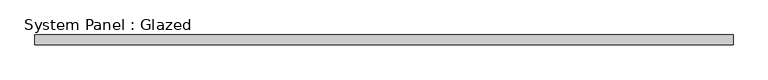
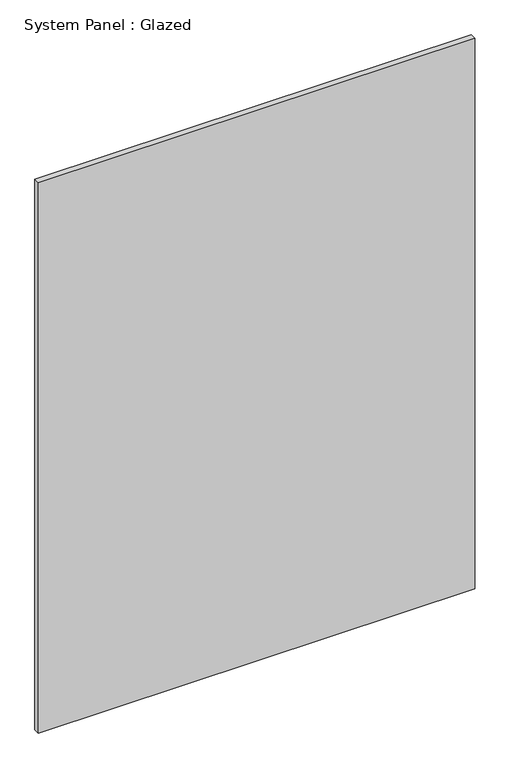
"""IFC4 building model written with IfcOpenShell, lengths in millimetres: plate geometry, System Panel : Glazed."""

from ifc_helpers import new_model, si_unit, origin, origin_with_axes, place, context, project, spatial, polyline, outline, extrude, source, transform, mapped, element, save


def system_panel_glazed_a143568c(model_context):
    return source(origin(), model_context, "Body", "SweptSolid", [
        extrude(outline(polyline([(914.4, 19.05), (-914.4, 19.05), (-914.4, 44.45), (914.4, 44.45), (914.4, 19.05)])), origin_with_axes(), (0.0, 0.0, 1.0), 2438.4),
    ])


if __name__ == "__main__":
    model = new_model("IFC4")
    model_context = context("Model", 3, world=origin())
    ifc_project = project(units=[si_unit("LENGTHUNIT", "METRE", prefix="MILLI")], contexts=[model_context])
    site = spatial("IfcSite", under=ifc_project)
    building = spatial("IfcBuilding", under=site)
    placement = place(None, origin())
    system_panel_glazed_shape = system_panel_glazed_a143568c(model_context)
    element("IfcPlate", 1, ObjectType="System Panel : Glazed", at=placement, inside=building, context=model_context, shape_type="MappedRepresentation", body=[
        mapped(system_panel_glazed_shape, transform((0.0, 0.0, 0.0), x_axis=(1.0, 0.0, 0.0), y_axis=(0.0, 1.0, 0.0), z_axis=(0.0, 0.0, 1.0))),
    ])
    save(model, "model.ifc")

# Revit data of these elements
# Type "System Panel : Glazed"
#   Construction Type Id = "GSP4R"
#   Analytic Construction = "1/8 in Pilkington single glazing"
#   Visual Light Transmittance = 0.9
#   Solar Heat Gain Coefficient = 0.86
#   Heat Transfer Coefficient (U) = 1.18115 BTU/(h·ft²·°F)
# Element 1 (IfcPlate, "System Panel : Glazed")
#   Materials on its faces: "Glass"
# Materials
#   "Glass": class "Glass", colour RGB 0 128 192, transparency 0.75, Description = "Soda Lime Glass", Cost = 0
